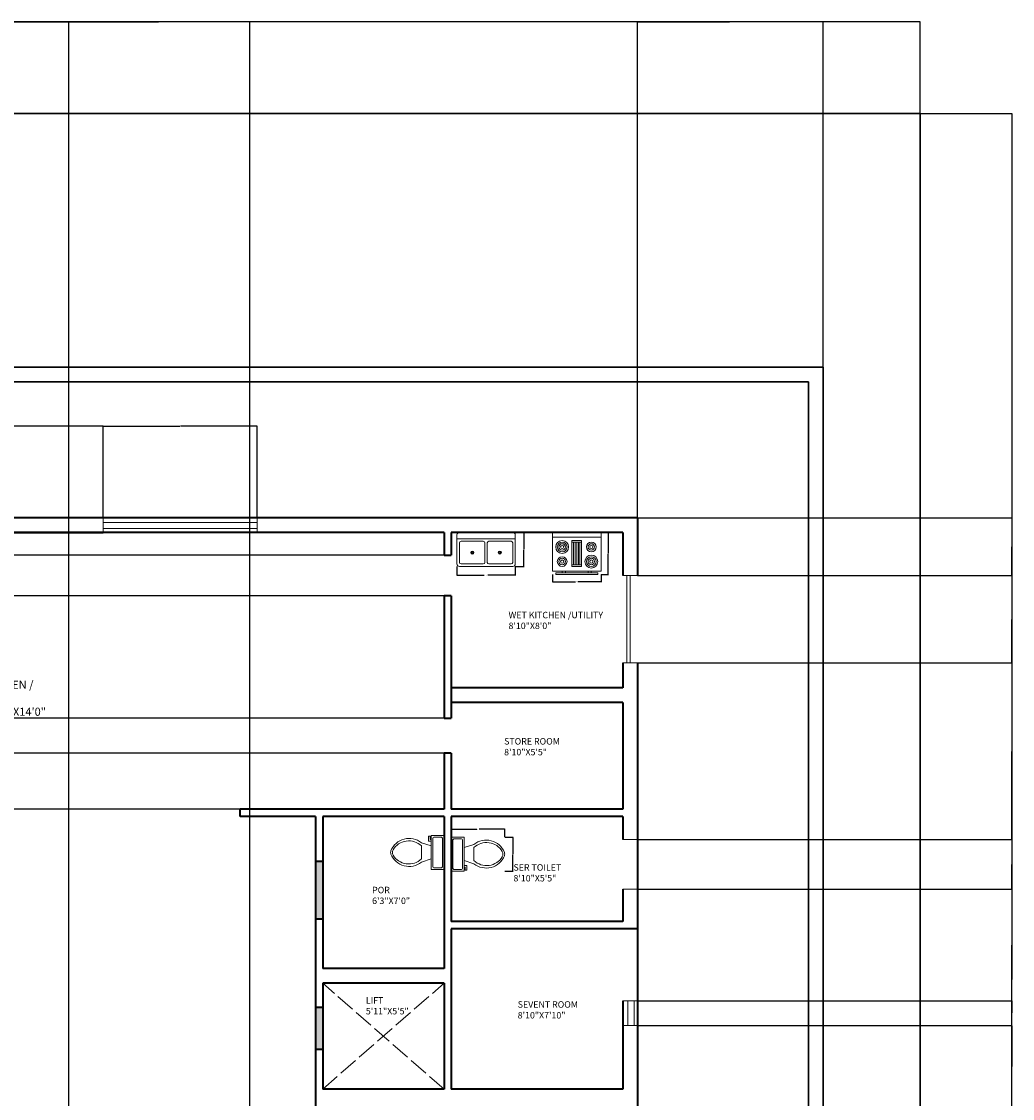
# Model space of a CAD drawing. Units: inches. Extents: x 727 to 1967, y -579 to 606.
# Tile 5 of 5: x 1355 to 1967, y -60 to 606. Entities that reach past the tile are written whole.
import ezdxf

# ---------------------------------------------------------------- set-up
doc = ezdxf.new("R2010")
doc.units = ezdxf.units.IN
doc.header["$MEASUREMENT"] = 0
doc.linetypes.add('ACAD_ISO02W100', pattern=[15, 12, -3])
for name, color, linetype, lineweight in [('A-ANNO-DIMS', 2, 'Continuous', 18), ('A-AREA-IDEN', 7, 'Continuous', 18), ('A-EQPM', 8, 'Continuous', 18), ('A-FLOR-EVTR', 8, 'ACAD_ISO02W100', 18), ('A-FLOR-FIXT', 9, 'Continuous', 18), ('A-GLAZ', 4, 'Continuous', 18), ('A-WALL', 7, 'Continuous', 35), ('A-WALL-PATT', 9, 'Continuous', 13), ('C-PROP', 7, 'Continuous', 30)]:
    doc.layers.add(name, color=color, linetype=linetype, lineweight=lineweight)
doc.styles.get("Standard").update_dxf_attribs({"font": 'arial.ttf'})
doc.dimstyles.get("Standard").update_dxf_attribs({"dimtxt": 0.18, "dimasz": 0.18, "dimexe": 0.18, "dimexo": 0.0625, "dimgap": 0.09, "dimtad": 0, "dimtih": 1, "dimtoh": 1, "dimdec": 4, "dimzin": 0, "dimdsep": 46, "dimtxsty": 'Standard', "dimcen": 0.09, "dimadec": 0, "dimazin": 0, "dimtfac": 1, "dimtdec": 4, "dimtofl": 0, "dimtmove": 0, "dimatfit": 3, "dimfxl": 1, "dimtolj": 1, "dimtzin": 0, "dimarcsym": 0})

# ---------------------------------------------------------------- blocks, each defined once
blk = doc.blocks.new('Range-Oven - 30 in top')
for p, q in [((0, -3), (30, -3)), ((12, -6), (18, -6)), ((13, -20), (13, -6)), ((14, -6), (14, -20)), ((15, -20), (15, -6)), ((16, -6), (16, -20)), ((17, -20), (17, -6)), ((6, -24), (6, -25)), ((8, -25), (8, -24)), ((18, -20), (12, -20)), ((22, -25), (22, -24)), ((24, -24), (24, -25))]:
    blk.add_line(p, q)
for points in [[(0, -24), (0, 0), (30, 0), (30, -24)], [(12, -21), (12, -5), (18, -5), (18, -21)], [(2, -26), (2, -25), (28, -25), (28, -26)]]:
    blk.add_lwpolyline(points, close=True)
for centre, radius in [((6, -9), 4), ((6, -9), 3), ((24, -9), 3), ((6, -9), 2), ((6, -9), 1), ((24, -9), 2), ((24, -9), 1), ((6, -18), 3), ((6, -18), 2), ((6, -18), 1), ((24, -18), 4), ((24, -18), 3), ((24, -18), 2), ((24, -18), 1)]:
    blk.add_circle(centre, radius)
blk = doc.blocks.new('Sink-double - 36 in top')
for p, q in [((-18, -4), (18, -4)), ((-0.75, -18.5), (-0.75, -6.5)), ((0.75, -6.5), (0.75, -18.5))]:
    blk.add_line(p, q)
for points in [[(-16.5, 0), (16.5, 0)], [(-18, -19.5), (-18, -1.5)], [(-16.5, -18.5), (-16.5, -6.5)], [(-15.5, -5.5), (-1.75, -5.5)], [(1.75, -5.5), (15.5, -5.5)], [(16.5, -6.5), (16.5, -18.5)], [(18, -1.5), (18, -19.5)], [(-1.75, -19.5), (-15.5, -19.5)], [(15.5, -19.5), (1.75, -19.5)], [(16.5, -21), (-16.5, -21)]]:
    blk.add_lwpolyline(points)
for centre, radius in [((-8.5, -12.5), 1), ((-8.5, -12.5), 0.5), ((8.5, -12.5), 1), ((8.5, -12.5), 0.5)]:
    blk.add_circle(centre, radius)
for centre, radius, start, end in [((-16.5, -1.5), 1.5, 90, 180), ((16.5, -1.5), 1.5, 0, 90), ((-15.5, -6.5), 1, 90, 180), ((-1.75, -6.5), 1, 0, 90), ((1.75, -6.5), 1, 90, 180), ((15.5, -6.5), 1, 0, 90), ((-16.5, -19.5), 1.5, 180, 270), ((-15.5, -18.5), 1, 180, 270), ((-1.75, -18.5), 1, 270, 0), ((1.75, -18.5), 1, 180, 270), ((15.5, -18.5), 1, 270, 0), ((16.5, -19.5), 1.5, 270, 0)]:
    blk.add_arc(centre, radius, start, end)
blk = doc.blocks.new('Toilet - top')
for p, q in [((9.5, -6), (9.5, -2)), ((-10, -8.5), (-8, -8.5)), ((-10, -9.5), (-10, -8.5)), ((-7, -9.5), (-10, -9.5)), ((-8, -8.5), (-8, -8)), ((-7, -8), (-7, -9.5)), ((-4, -8), (-6, -14)), ((4, -8), (6, -14)), ((4, -14), (-4, -14))]:
    blk.add_line(p, q)
blk.add_lwpolyline([(10.5, -8), (10.5, 0), (-10.5, 0), (-10.5, -8)], close=True)
for points in [[(-9.5, -2), (-9.5, -6)], [(8.5, -1), (-8.5, -1)], [(-8.5, -7), (8.5, -7)]]:
    blk.add_lwpolyline(points)
for centre, radius, start, end in [((-8.62, -1.88), 0.884, 81.8699, 188.1301), ((-8.62, -6.12), 0.884, 171.8699, 278.1301), ((8.62, -1.88), 0.884, 351.8699, 98.1301), ((8.62, -6.12), 0.884, 261.8699, 8.1301), ((3.52, -21.58), 12.17, 141.46911, 247.97143), ((4.2, -21.82), 11.33, 136.36773, 238.94682), ((-3.52, -21.58), 12.17, 292.02843, 38.53071), ((-4.2, -21.82), 11.33, 301.05301, 43.63209), ((0, -27.88), 4, 245.73182, 294.26817), ((0, -29), 4, 254.86053, 285.13947)]:
    blk.add_arc(centre, radius, start, end)
blk = doc.blocks.new('*D20')
at = {"layer": 'A-ANNO-DIMS', "color": 0, "lineweight": -2, "transparency": 16777216}
for p, q in [((1620.35, 101.83), (1620.35, 106.91)), ((1620.53, 106.73), (1636.09, 106.73)), ((1653.21, 106.73), (1637.65, 106.73)), ((1653.39, 101.83), (1653.39, 106.91))]:
    blk.add_line(p, q, dxfattribs=at)
at = {"layer": 'A-ANNO-DIMS', "color": 0, "transparency": 16777216}
for points in [[(1620.53, 106.76), (1620.53, 106.7), (1620.35, 106.73)], [(1653.21, 106.76), (1653.21, 106.7), (1653.39, 106.73)]]:
    blk.add_solid(points, dxfattribs=at)
at = {"layer": 'Defpoints', "color": 0, "transparency": 16777216}
for p in [(1620.35, 106.73), (1620.35, 101.77), (1653.39, 101.77)]:
    blk.add_point(p, dxfattribs=at)
at = {"layer": 'A-ANNO-DIMS', "color": 0, "transparency": 16777216, "insert": (1636.87, 106.73), "char_height": 0.18, "attachment_point": 5}
blk.add_mtext('\\A1;WC 33 TYP.', dxfattribs=at)
blk = doc.blocks.new('*D21')
at = {"layer": 'A-ANNO-DIMS', "color": 0, "lineweight": -2, "transparency": 16777216}
for p, q in [((1653.46, 101.77), (1658.53, 101.77)), ((1658.35, 101.59), (1658.35, 91.45)), ((1658.35, 80.95), (1658.35, 91.09)), ((1653.46, 80.77), (1658.53, 80.77))]:
    blk.add_line(p, q, dxfattribs=at)
at = {"layer": 'A-ANNO-DIMS', "color": 0, "transparency": 16777216}
for points in [[(1658.32, 101.59), (1658.38, 101.59), (1658.35, 101.77)], [(1658.32, 80.95), (1658.38, 80.95), (1658.35, 80.77)]]:
    blk.add_solid(points, dxfattribs=at)
at = {"layer": 'Defpoints', "color": 0, "transparency": 16777216}
for p in [(1653.39, 101.77), (1658.35, 101.77), (1653.39, 80.77)]:
    blk.add_point(p, dxfattribs=at)
at = {"layer": 'A-ANNO-DIMS', "color": 0, "transparency": 16777216, "insert": (1658.35, 91.27), "char_height": 0.18, "attachment_point": 5}
blk.add_mtext('\\A1;21 TYP.', dxfattribs=at)
blk = doc.blocks.new('*D28')
at = {"layer": 'A-ANNO-DIMS', "color": 0, "lineweight": -2, "transparency": 16777216}
for p, q in [((1682.86, 263.95), (1682.86, 259.34)), ((1683.04, 259.52), (1697.17, 259.52)), ((1712.68, 259.52), (1698.56, 259.52)), ((1712.86, 263.95), (1712.86, 259.34))]:
    blk.add_line(p, q, dxfattribs=at)
at = {"layer": 'A-ANNO-DIMS', "color": 0, "transparency": 16777216}
for points in [[(1683.04, 259.55), (1683.04, 259.49), (1682.86, 259.52)], [(1712.68, 259.55), (1712.68, 259.49), (1712.86, 259.52)]]:
    blk.add_solid(points, dxfattribs=at)
at = {"layer": 'Defpoints', "color": 0, "transparency": 16777216}
for p in [(1682.86, 264.02), (1712.86, 264.02), (1712.86, 259.52)]:
    blk.add_point(p, dxfattribs=at)
at = {"layer": 'A-ANNO-DIMS', "color": 0, "transparency": 16777216, "insert": (1697.86, 259.52), "char_height": 0.18, "attachment_point": 5}
blk.add_mtext('\\A1;RANGE 30', dxfattribs=at)
blk = doc.blocks.new('*D29')
at = {"layer": 'A-ANNO-DIMS', "color": 0, "lineweight": -2, "transparency": 16777216}
for p, q in [((1712.93, 290.02), (1717.54, 290.02)), ((1717.36, 289.84), (1717.36, 277.2)), ((1717.36, 264.2), (1717.36, 276.83)), ((1712.93, 264.02), (1717.54, 264.02))]:
    blk.add_line(p, q, dxfattribs=at)
at = {"layer": 'A-ANNO-DIMS', "color": 0, "transparency": 16777216}
for points in [[(1717.33, 289.84), (1717.39, 289.84), (1717.36, 290.02)], [(1717.33, 264.2), (1717.39, 264.2), (1717.36, 264.02)]]:
    blk.add_solid(points, dxfattribs=at)
at = {"layer": 'Defpoints', "color": 0, "transparency": 16777216}
for p in [(1712.86, 290.02), (1717.36, 290.02), (1712.86, 264.02)]:
    blk.add_point(p, dxfattribs=at)
at = {"layer": 'A-ANNO-DIMS', "color": 0, "transparency": 16777216, "insert": (1717.36, 277.02), "char_height": 0.18, "attachment_point": 5}
blk.add_mtext('\\A1;26', dxfattribs=at)
blk = doc.blocks.new('*D30')
at = {"layer": 'A-ANNO-DIMS', "color": 0, "lineweight": -2, "transparency": 16777216}
for p, q in [((1623.85, 268.95), (1623.85, 263.44)), ((1659.85, 268.95), (1659.85, 263.44)), ((1624.03, 263.62), (1640.75, 263.62)), ((1659.67, 263.62), (1642.94, 263.62))]:
    blk.add_line(p, q, dxfattribs=at)
at = {"layer": 'A-ANNO-DIMS', "color": 0, "transparency": 16777216}
for points in [[(1624.03, 263.65), (1624.03, 263.59), (1623.85, 263.62)], [(1659.67, 263.65), (1659.67, 263.59), (1659.85, 263.62)]]:
    blk.add_solid(points, dxfattribs=at)
at = {"layer": 'Defpoints', "color": 0, "transparency": 16777216}
for p in [(1623.85, 269.02), (1659.85, 269.02), (1659.85, 263.62)]:
    blk.add_point(p, dxfattribs=at)
at = {"layer": 'A-ANNO-DIMS', "color": 0, "transparency": 16777216, "insert": (1641.85, 263.62), "char_height": 0.18, "attachment_point": 5}
blk.add_mtext('\\A1;DOUBLE SINK 36', dxfattribs=at)
blk = doc.blocks.new('*D31')
at = {"layer": 'A-ANNO-DIMS', "color": 0, "lineweight": -2, "transparency": 16777216}
for p, q in [((1659.91, 290.02), (1665.43, 290.02)), ((1665.25, 289.84), (1665.25, 279.7)), ((1665.25, 269.2), (1665.25, 279.33)), ((1659.91, 269.02), (1665.43, 269.02))]:
    blk.add_line(p, q, dxfattribs=at)
at = {"layer": 'A-ANNO-DIMS', "color": 0, "transparency": 16777216}
for points in [[(1665.22, 289.84), (1665.28, 289.84), (1665.25, 290.02)], [(1665.22, 269.2), (1665.28, 269.2), (1665.25, 269.02)]]:
    blk.add_solid(points, dxfattribs=at)
at = {"layer": 'Defpoints', "color": 0, "transparency": 16777216}
for p in [(1659.85, 290.02), (1665.25, 290.02), (1659.85, 269.02)]:
    blk.add_point(p, dxfattribs=at)
at = {"layer": 'A-ANNO-DIMS', "color": 0, "transparency": 16777216, "insert": (1665.25, 279.52), "char_height": 0.18, "attachment_point": 5}
blk.add_mtext('\\A1;21', dxfattribs=at)
blk = doc.blocks.new('*D38')
at = {"layer": 'A-ANNO-DIMS', "color": 0, "lineweight": -2, "transparency": 16777216}
for p, q in [((783.58, 548.95), (783.58, 605.67)), ((1910.18, 548.95), (1910.18, 605.67)), ((783.76, 605.49), (1346.42, 605.49)), ((1910, 605.49), (1347.33, 605.49))]:
    blk.add_line(p, q, dxfattribs=at)
at = {"layer": 'A-ANNO-DIMS', "color": 0, "transparency": 16777216}
for points in [[(783.76, 605.52), (783.76, 605.46), (783.58, 605.49)], [(1910, 605.52), (1910, 605.46), (1910.18, 605.49)]]:
    blk.add_solid(points, dxfattribs=at)
at = {"layer": 'Defpoints', "color": 0, "transparency": 16777216}
for p in [(1910.18, 605.49), (783.58, 548.89), (1910.18, 548.89)]:
    blk.add_point(p, dxfattribs=at)
at = {"layer": 'A-ANNO-DIMS', "color": 0, "transparency": 16777216, "insert": (1346.88, 605.49), "char_height": 0.18, "attachment_point": 5}
blk.add_mtext('\\A1;1126.6', dxfattribs=at)
blk = doc.blocks.new('*D39')
at = {"layer": 'A-ANNO-DIMS', "color": 0, "lineweight": -2, "transparency": 16777216}
for p, q in [((1910.24, 548.89), (1966.96, 548.89)), ((1966.78, 548.71), (1966.78, 13.72)), ((1966.78, -521.63), (1966.78, 13.36)), ((1910.24, -521.81), (1966.96, -521.81))]:
    blk.add_line(p, q, dxfattribs=at)
at = {"layer": 'A-ANNO-DIMS', "color": 0, "transparency": 16777216}
for points in [[(1966.75, 548.71), (1966.81, 548.71), (1966.78, 548.89)], [(1966.75, -521.63), (1966.81, -521.63), (1966.78, -521.81)]]:
    blk.add_solid(points, dxfattribs=at)
at = {"layer": 'Defpoints', "color": 0, "transparency": 16777216}
for p in [(1910.18, 548.89), (1966.78, 548.89), (1910.18, -521.81)]:
    blk.add_point(p, dxfattribs=at)
at = {"layer": 'A-ANNO-DIMS', "color": 0, "transparency": 16777216, "insert": (1966.78, 13.54), "char_height": 0.18, "attachment_point": 5}
blk.add_mtext('\\A1;1070.7', dxfattribs=at)
blk = doc.blocks.new('*D42')
at = {"layer": 'A-ANNO-DIMS', "color": 0, "lineweight": -2, "transparency": 16777216}
for p, q in [((1099.85, 299.08), (1099.85, 605.67)), ((1735.35, 299.08), (1735.35, 605.67)), ((1100.03, 605.49), (1417.2, 605.49)), ((1735.17, 605.49), (1417.99, 605.49))]:
    blk.add_line(p, q, dxfattribs=at)
at = {"layer": 'A-ANNO-DIMS', "color": 0, "transparency": 16777216}
for points in [[(1100.03, 605.52), (1100.03, 605.46), (1099.85, 605.49)], [(1735.17, 605.52), (1735.17, 605.46), (1735.35, 605.49)]]:
    blk.add_solid(points, dxfattribs=at)
at = {"layer": 'Defpoints', "color": 0, "transparency": 16777216}
for p in [(1735.35, 605.49), (1099.85, 299.02), (1735.35, 299.02)]:
    blk.add_point(p, dxfattribs=at)
at = {"layer": 'A-ANNO-DIMS', "color": 0, "transparency": 16777216, "insert": (1417.6, 605.49), "char_height": 0.18, "attachment_point": 5}
blk.add_mtext('\\A1;635.5', dxfattribs=at)
blk = doc.blocks.new('*D43')
at = {"layer": 'A-ANNO-DIMS', "color": 0, "lineweight": -2, "transparency": 16777216}
for p, q in [((1735.35, 299.08), (1735.35, 605.67)), ((1850.18, 392.08), (1850.18, 605.67)), ((1735.53, 605.49), (1792.31, 605.49)), ((1850, 605.49), (1793.22, 605.49))]:
    blk.add_line(p, q, dxfattribs=at)
at = {"layer": 'A-ANNO-DIMS', "color": 0, "transparency": 16777216}
for points in [[(1735.53, 605.52), (1735.53, 605.46), (1735.35, 605.49)], [(1850, 605.52), (1850, 605.46), (1850.18, 605.49)]]:
    blk.add_solid(points, dxfattribs=at)
at = {"layer": 'Defpoints', "color": 0, "transparency": 16777216}
for p in [(1850.18, 605.49), (1850.18, 392.02), (1735.35, 299.02)]:
    blk.add_point(p, dxfattribs=at)
at = {"layer": 'A-ANNO-DIMS', "color": 0, "transparency": 16777216, "insert": (1792.76, 605.49), "char_height": 0.18, "attachment_point": 5}
blk.add_mtext('\\A1;114.83', dxfattribs=at)
blk = doc.blocks.new('*D57')
at = {"layer": 'A-ANNO-DIMS', "color": 0, "lineweight": -2, "transparency": 16777216}
for p, q in [((1288.64, 299.08), (1288.64, 355.8)), ((1288.82, 355.62), (1346.51, 355.62)), ((1405.1, 355.62), (1347.42, 355.62)), ((1405.28, 299.08), (1405.28, 355.8))]:
    blk.add_line(p, q, dxfattribs=at)
at = {"layer": 'A-ANNO-DIMS', "color": 0, "transparency": 16777216}
for points in [[(1288.82, 355.65), (1288.82, 355.59), (1288.64, 355.62)], [(1405.1, 355.65), (1405.1, 355.59), (1405.28, 355.62)]]:
    blk.add_solid(points, dxfattribs=at)
at = {"layer": 'Defpoints', "color": 0, "transparency": 16777216}
for p in [(1405.28, 355.62), (1288.64, 299.02), (1405.28, 299.02)]:
    blk.add_point(p, dxfattribs=at)
at = {"layer": 'A-ANNO-DIMS', "color": 0, "transparency": 16777216, "insert": (1346.96, 355.62), "char_height": 0.18, "attachment_point": 5}
blk.add_mtext('\\A1;116.65', dxfattribs=at)
blk = doc.blocks.new('*D58')
at = {"layer": 'A-ANNO-DIMS', "color": 0, "lineweight": -2, "transparency": 16777216}
for p, q in [((1405.28, 299.08), (1405.28, 355.8)), ((1405.46, 355.62), (1452.56, 355.62)), ((1500.1, 355.62), (1453, 355.62)), ((1500.28, 299.08), (1500.28, 355.8))]:
    blk.add_line(p, q, dxfattribs=at)
at = {"layer": 'A-ANNO-DIMS', "color": 0, "transparency": 16777216}
for points in [[(1405.46, 355.65), (1405.46, 355.59), (1405.28, 355.62)], [(1500.1, 355.65), (1500.1, 355.59), (1500.28, 355.62)]]:
    blk.add_solid(points, dxfattribs=at)
at = {"layer": 'Defpoints', "color": 0, "transparency": 16777216}
for p in [(1500.28, 355.62), (1405.28, 299.02), (1500.28, 299.02)]:
    blk.add_point(p, dxfattribs=at)
at = {"layer": 'A-ANNO-DIMS', "color": 0, "transparency": 16777216, "insert": (1452.78, 355.62), "char_height": 0.18, "attachment_point": 5}
blk.add_mtext('\\A1;95', dxfattribs=at)
blk = doc.blocks.new('*D60')
at = {"layer": 'A-ANNO-DIMS', "color": 0, "lineweight": -2, "transparency": 16777216}
for p, q in [((1383.91, -185.42), (1383.91, 605.67)), ((1495.93, -185.42), (1495.93, 605.67)), ((1384.09, 605.49), (1439.47, 605.49)), ((1495.75, 605.49), (1440.38, 605.49))]:
    blk.add_line(p, q, dxfattribs=at)
at = {"layer": 'A-ANNO-DIMS', "color": 0, "transparency": 16777216}
for points in [[(1384.09, 605.52), (1384.09, 605.46), (1383.91, 605.49)], [(1495.75, 605.52), (1495.75, 605.46), (1495.93, 605.49)]]:
    blk.add_solid(points, dxfattribs=at)
at = {"layer": 'Defpoints', "color": 0, "transparency": 16777216}
for p in [(1495.93, 605.49), (1383.91, -185.48), (1495.93, -185.48)]:
    blk.add_point(p, dxfattribs=at)
at = {"layer": 'A-ANNO-DIMS', "color": 0, "transparency": 16777216, "insert": (1439.92, 605.49), "char_height": 0.18, "attachment_point": 5}
blk.add_mtext('\\A1;112.02', dxfattribs=at)
blk = doc.blocks.new('*D61')
at = {"layer": 'A-ANNO-DIMS', "color": 0, "lineweight": -2, "transparency": 16777216}
for p, q in [((1735.41, 299.02), (1966.96, 299.02)), ((1966.78, 298.84), (1966.78, 281.43)), ((1966.78, 263.66), (1966.78, 281.07)), ((1735.41, 263.48), (1966.96, 263.48))]:
    blk.add_line(p, q, dxfattribs=at)
at = {"layer": 'A-ANNO-DIMS', "color": 0, "transparency": 16777216}
for points in [[(1966.75, 298.84), (1966.81, 298.84), (1966.78, 299.02)], [(1966.75, 263.66), (1966.81, 263.66), (1966.78, 263.48)]]:
    blk.add_solid(points, dxfattribs=at)
at = {"layer": 'Defpoints', "color": 0, "transparency": 16777216}
for p in [(1735.35, 299.02), (1735.35, 263.48), (1966.78, 263.48)]:
    blk.add_point(p, dxfattribs=at)
at = {"layer": 'A-ANNO-DIMS', "color": 0, "transparency": 16777216, "insert": (1966.78, 281.25), "char_height": 0.18, "attachment_point": 5}
blk.add_mtext('\\A1;35.534', dxfattribs=at)
blk = doc.blocks.new('*D62')
at = {"layer": 'A-ANNO-DIMS', "color": 0, "lineweight": -2, "transparency": 16777216}
for p, q in [((1735.41, 263.48), (1966.96, 263.48)), ((1966.78, 263.3), (1966.78, 236.6)), ((1966.78, 209.53), (1966.78, 236.24)), ((1735.41, 209.35), (1966.96, 209.35))]:
    blk.add_line(p, q, dxfattribs=at)
at = {"layer": 'A-ANNO-DIMS', "color": 0, "transparency": 16777216}
for points in [[(1966.75, 263.3), (1966.81, 263.3), (1966.78, 263.48)], [(1966.75, 209.53), (1966.81, 209.53), (1966.78, 209.35)]]:
    blk.add_solid(points, dxfattribs=at)
at = {"layer": 'Defpoints', "color": 0, "transparency": 16777216}
for p in [(1735.35, 263.48), (1735.35, 209.35), (1966.78, 209.35)]:
    blk.add_point(p, dxfattribs=at)
at = {"layer": 'A-ANNO-DIMS', "color": 0, "transparency": 16777216, "insert": (1966.78, 236.42), "char_height": 0.18, "attachment_point": 5}
blk.add_mtext('\\A1;54.13', dxfattribs=at)
blk = doc.blocks.new('*D63')
at = {"layer": 'A-ANNO-DIMS', "color": 0, "lineweight": -2, "transparency": 16777216}
for p, q in [((1735.41, 209.35), (1966.96, 209.35)), ((1966.78, 209.17), (1966.78, 155.02)), ((1966.78, 100.51), (1966.78, 154.66)), ((1735.41, 100.33), (1966.96, 100.33))]:
    blk.add_line(p, q, dxfattribs=at)
at = {"layer": 'A-ANNO-DIMS', "color": 0, "transparency": 16777216}
for points in [[(1966.75, 209.17), (1966.81, 209.17), (1966.78, 209.35)], [(1966.75, 100.51), (1966.81, 100.51), (1966.78, 100.33)]]:
    blk.add_solid(points, dxfattribs=at)
at = {"layer": 'Defpoints', "color": 0, "transparency": 16777216}
for p in [(1735.35, 209.35), (1735.35, 100.33), (1966.78, 100.33)]:
    blk.add_point(p, dxfattribs=at)
at = {"layer": 'A-ANNO-DIMS', "color": 0, "transparency": 16777216, "insert": (1966.78, 154.84), "char_height": 0.18, "attachment_point": 5}
blk.add_mtext('\\A1;109.03', dxfattribs=at)
blk = doc.blocks.new('*D64')
at = {"layer": 'A-ANNO-DIMS', "color": 0, "lineweight": -2, "transparency": 16777216}
for p, q in [((1735.41, 100.33), (1966.96, 100.33)), ((1966.78, 100.15), (1966.78, 85.17)), ((1966.78, 69.83), (1966.78, 84.81)), ((1735.41, 69.65), (1966.96, 69.65))]:
    blk.add_line(p, q, dxfattribs=at)
at = {"layer": 'A-ANNO-DIMS', "color": 0, "transparency": 16777216}
for points in [[(1966.75, 100.15), (1966.81, 100.15), (1966.78, 100.33)], [(1966.75, 69.83), (1966.81, 69.83), (1966.78, 69.65)]]:
    blk.add_solid(points, dxfattribs=at)
at = {"layer": 'Defpoints', "color": 0, "transparency": 16777216}
for p in [(1735.35, 100.33), (1735.35, 69.65), (1966.78, 69.65)]:
    blk.add_point(p, dxfattribs=at)
at = {"layer": 'A-ANNO-DIMS', "color": 0, "transparency": 16777216, "insert": (1966.78, 84.99), "char_height": 0.18, "attachment_point": 5}
blk.add_mtext('\\A1;30.67', dxfattribs=at)
blk = doc.blocks.new('*D65')
at = {"layer": 'A-ANNO-DIMS', "color": 0, "lineweight": -2, "transparency": 16777216}
for p, q in [((1735.41, 69.65), (1966.96, 69.65)), ((1966.78, 69.47), (1966.78, 35.35)), ((1966.78, 0.87), (1966.78, 34.99)), ((1735.41, 0.69), (1966.96, 0.69))]:
    blk.add_line(p, q, dxfattribs=at)
at = {"layer": 'A-ANNO-DIMS', "color": 0, "transparency": 16777216}
for points in [[(1966.75, 69.47), (1966.81, 69.47), (1966.78, 69.65)], [(1966.75, 0.87), (1966.81, 0.87), (1966.78, 0.69)]]:
    blk.add_solid(points, dxfattribs=at)
at = {"layer": 'Defpoints', "color": 0, "transparency": 16777216}
for p in [(1735.35, 69.65), (1735.35, 0.69), (1966.78, 0.69)]:
    blk.add_point(p, dxfattribs=at)
at = {"layer": 'A-ANNO-DIMS', "color": 0, "transparency": 16777216, "insert": (1966.78, 35.17), "char_height": 0.18, "attachment_point": 5}
blk.add_mtext('\\A1;68.97', dxfattribs=at)
blk = doc.blocks.new('*D66')
at = {"layer": 'A-ANNO-DIMS', "color": 0, "lineweight": -2, "transparency": 16777216}
for p, q in [((1735.41, 0.69), (1966.96, 0.69)), ((1966.78, 0.51), (1966.78, -6.85)), ((1966.78, -14.57), (1966.78, -7.22)), ((1735.41, -14.75), (1966.96, -14.75))]:
    blk.add_line(p, q, dxfattribs=at)
at = {"layer": 'A-ANNO-DIMS', "color": 0, "transparency": 16777216}
for points in [[(1966.75, 0.51), (1966.81, 0.51), (1966.78, 0.69)], [(1966.75, -14.57), (1966.81, -14.57), (1966.78, -14.75)]]:
    blk.add_solid(points, dxfattribs=at)
at = {"layer": 'Defpoints', "color": 0, "transparency": 16777216}
for p in [(1735.35, 0.69), (1735.35, -14.75), (1966.78, -14.75)]:
    blk.add_point(p, dxfattribs=at)
at = {"layer": 'A-ANNO-DIMS', "color": 0, "transparency": 16777216, "insert": (1966.78, -7.03), "char_height": 0.18, "attachment_point": 5}
blk.add_mtext('\\A1;15.44', dxfattribs=at)
blk = doc.blocks.new('*D67')
at = {"layer": 'A-ANNO-DIMS', "color": 0, "lineweight": -2, "transparency": 16777216}
for p, q in [((1735.41, -14.75), (1966.96, -14.75)), ((1966.78, -14.93), (1966.78, -39.94)), ((1966.78, -65.3), (1966.78, -40.3)), ((1735.41, -65.48), (1966.96, -65.48))]:
    blk.add_line(p, q, dxfattribs=at)
at = {"layer": 'A-ANNO-DIMS', "color": 0, "transparency": 16777216}
for points in [[(1966.75, -14.93), (1966.81, -14.93), (1966.78, -14.75)], [(1966.75, -65.3), (1966.81, -65.3), (1966.78, -65.48)]]:
    blk.add_solid(points, dxfattribs=at)
at = {"layer": 'Defpoints', "color": 0, "transparency": 16777216}
for p in [(1735.35, -14.75), (1735.35, -65.48), (1966.78, -65.48)]:
    blk.add_point(p, dxfattribs=at)
at = {"layer": 'A-ANNO-DIMS', "color": 0, "transparency": 16777216, "insert": (1966.78, -40.12), "char_height": 0.18, "attachment_point": 5}
blk.add_mtext('\\A1;50.73', dxfattribs=at)
blk = doc.blocks.new('*D69')
at = {"layer": 'A-ANNO-DIMS', "color": 0, "lineweight": -2, "transparency": 16777216}
for p, q in [((1615.78, 290.02), (726.8, 290.02)), ((726.98, 289.84), (726.98, 283.18)), ((726.98, 276.17), (726.98, 282.82)), ((1615.78, 275.99), (726.8, 275.99))]:
    blk.add_line(p, q, dxfattribs=at)
at = {"layer": 'A-ANNO-DIMS', "color": 0, "transparency": 16777216}
for points in [[(726.95, 289.84), (727.01, 289.84), (726.98, 290.02)], [(726.95, 276.17), (727.01, 276.17), (726.98, 275.99)]]:
    blk.add_solid(points, dxfattribs=at)
at = {"layer": 'Defpoints', "color": 0, "transparency": 16777216}
for p in [(1615.85, 290.02), (726.98, 275.99), (1615.85, 275.99)]:
    blk.add_point(p, dxfattribs=at)
at = {"layer": 'A-ANNO-DIMS', "color": 0, "transparency": 16777216, "insert": (726.98, 283), "char_height": 0.18, "attachment_point": 5}
blk.add_mtext('\\A1;14.027', dxfattribs=at)
blk = doc.blocks.new('*D70')
at = {"layer": 'A-ANNO-DIMS', "color": 0, "lineweight": -2, "transparency": 16777216}
for p, q in [((1615.78, 275.99), (726.8, 275.99)), ((726.98, 275.81), (726.98, 263.6)), ((726.98, 251.03), (726.98, 263.24)), ((1615.78, 250.85), (726.8, 250.85))]:
    blk.add_line(p, q, dxfattribs=at)
at = {"layer": 'A-ANNO-DIMS', "color": 0, "transparency": 16777216}
for points in [[(726.95, 275.81), (727.01, 275.81), (726.98, 275.99)], [(726.95, 251.03), (727.01, 251.03), (726.98, 250.85)]]:
    blk.add_solid(points, dxfattribs=at)
at = {"layer": 'Defpoints', "color": 0, "transparency": 16777216}
for p in [(1615.85, 275.99), (726.98, 250.85), (1615.85, 250.85)]:
    blk.add_point(p, dxfattribs=at)
at = {"layer": 'A-ANNO-DIMS', "color": 0, "transparency": 16777216, "insert": (726.98, 263.42), "char_height": 0.18, "attachment_point": 5}
blk.add_mtext('\\A1;25.135', dxfattribs=at)
blk = doc.blocks.new('*D71')
at = {"layer": 'A-ANNO-DIMS', "color": 0, "lineweight": -2, "transparency": 16777216}
for p, q in [((1615.78, 250.85), (726.8, 250.85)), ((726.98, 250.67), (726.98, 213.22)), ((726.98, 175.39), (726.98, 212.85)), ((1615.78, 175.21), (726.8, 175.21))]:
    blk.add_line(p, q, dxfattribs=at)
at = {"layer": 'A-ANNO-DIMS', "color": 0, "transparency": 16777216}
for points in [[(726.95, 250.67), (727.01, 250.67), (726.98, 250.85)], [(726.95, 175.39), (727.01, 175.39), (726.98, 175.21)]]:
    blk.add_solid(points, dxfattribs=at)
at = {"layer": 'Defpoints', "color": 0, "transparency": 16777216}
for p in [(1615.85, 250.85), (726.98, 175.21), (1615.85, 175.21)]:
    blk.add_point(p, dxfattribs=at)
at = {"layer": 'A-ANNO-DIMS', "color": 0, "transparency": 16777216, "insert": (726.98, 213.03), "char_height": 0.18, "attachment_point": 5}
blk.add_mtext('\\A1;75.64', dxfattribs=at)
blk = doc.blocks.new('*D72')
at = {"layer": 'A-ANNO-DIMS', "color": 0, "lineweight": -2, "transparency": 16777216}
for p, q in [((1615.78, 175.21), (726.8, 175.21)), ((726.98, 175.03), (726.98, 164.56)), ((726.98, 153.73), (726.98, 164.2)), ((1615.78, 153.55), (726.8, 153.55))]:
    blk.add_line(p, q, dxfattribs=at)
at = {"layer": 'A-ANNO-DIMS', "color": 0, "transparency": 16777216}
for points in [[(726.95, 175.03), (727.01, 175.03), (726.98, 175.21)], [(726.95, 153.73), (727.01, 153.73), (726.98, 153.55)]]:
    blk.add_solid(points, dxfattribs=at)
at = {"layer": 'Defpoints', "color": 0, "transparency": 16777216}
for p in [(1615.85, 175.21), (726.98, 153.55), (1615.85, 153.55)]:
    blk.add_point(p, dxfattribs=at)
at = {"layer": 'A-ANNO-DIMS', "color": 0, "transparency": 16777216, "insert": (726.98, 164.38), "char_height": 0.18, "attachment_point": 5}
blk.add_mtext('\\A1;21.67', dxfattribs=at)
blk = doc.blocks.new('*D73')
at = {"layer": 'A-ANNO-DIMS', "color": 0, "lineweight": -2, "transparency": 16777216}
for p, q in [((1615.78, 153.55), (726.8, 153.55)), ((726.98, 153.37), (726.98, 136.46)), ((726.98, 119.2), (726.98, 136.1)), ((1615.78, 119.02), (726.8, 119.02))]:
    blk.add_line(p, q, dxfattribs=at)
at = {"layer": 'A-ANNO-DIMS', "color": 0, "transparency": 16777216}
for points in [[(726.95, 153.37), (727.01, 153.37), (726.98, 153.55)], [(726.95, 119.2), (727.01, 119.2), (726.98, 119.02)]]:
    blk.add_solid(points, dxfattribs=at)
at = {"layer": 'Defpoints', "color": 0, "transparency": 16777216}
for p in [(1615.85, 153.55), (726.98, 119.02), (1615.85, 119.02)]:
    blk.add_point(p, dxfattribs=at)
at = {"layer": 'A-ANNO-DIMS', "color": 0, "transparency": 16777216, "insert": (726.98, 136.28), "char_height": 0.18, "attachment_point": 5}
blk.add_mtext('\\A1;34.53', dxfattribs=at)

msp = doc.modelspace()

# ---------------------------------------------------------------- hatches: boundary and pattern name
at = {"layer": 'A-WALL-PATT'}
h = msp.add_hatch(color=256, dxfattribs=at)
h.dxf.hatch_style = 1
h.paths.add_polyline_path([(1536.3463, 51.1439), (1540.8463, 51.1439), (1540.8463, 86.7969), (1536.3463, 86.7969)])
h.paths.add_polyline_path([(1536.3463, -29.217), (1540.8463, -29.217), (1540.8463, -3.5401), (1536.3463, -3.5401)])

# ---------------------------------------------------------------- linework, layer by layer
at = {"layer": 'A-FLOR-EVTR'}
for p, q in [((1540.8463, -53.9849), (1615.8463, 11.5151)), ((1615.8463, -53.9849), (1540.8463, 11.5151))]:
    msp.add_line(p, q, dxfattribs=at)
at = {"layer": 'A-GLAZ'}
for p, q in [((1405.2835, 290.0151), (1405.2835, 299.0151)), ((1405.2835, 299.0151), (1500.2781, 299.0151)), ((1405.2835, 292.5171), (1405.2835, 296.1248)), ((1405.2835, 296.1248), (1500.2781, 296.1248)), ((1500.2781, 299.0151), (1500.2781, 290.0151)), ((1500.2781, 292.5171), (1405.2835, 292.5171)), ((1500.2781, 290.0151), (1500.2781, 292.5171)), ((1735.3463, 263.4809), (1726.3463, 263.4809)), ((1728.876, 263.4809), (1728.876, 209.3543)), ((1730.8463, 209.3543), (1730.8463, 263.4809)), ((1726.3463, 209.3543), (1735.3463, 209.3543)), ((1728.876, 209.3543), (1730.8463, 209.3543)), ((1726.3463, 100.3256), (1735.3463, 100.3256)), ((1735.3463, 100.3256), (1735.3463, 69.6534)), ((1735.3463, 69.6534), (1726.3463, 69.6534)), ((1735.3463, 0.6867), (1726.3463, 0.6867)), ((1726.3463, 0.6867), (1729.3906, 0.6867)), ((1729.3906, 0.6867), (1729.3906, -14.7535)), ((1733.3452, -14.7535), (1733.3452, 0.6867)), ((1733.3452, 0.6867), (1735.3463, 0.6867)), ((1726.3463, -14.7535), (1733.3452, -14.7535)), ((1733.3452, -14.7535), (1735.3463, -14.7535)), ((1735.3463, -14.7535), (1733.3452, -14.7535))]:
    msp.add_line(p, q, dxfattribs=at)
at = {"layer": 'A-WALL'}
for p, q in [((1735.3463, 299.0151), (1288.6382, 299.0151)), ((1735.3463, 299.0151), (1735.3463, 263.4809)), ((1615.8463, 290.0151), (1283.8463, 290.0151)), ((1345.2945, 290.0151), (1405.2835, 290.0151)), ((1615.8463, 290.0151), (1615.8463, 275.988)), ((1620.3463, 290.0151), (1620.3463, 275.988)), ((1726.3463, 290.0151), (1620.3463, 290.0151)), ((1726.3463, 290.0151), (1726.3463, 263.4809)), ((1615.8463, 275.988), (1620.3463, 275.988)), ((1620.3463, 250.8534), (1615.8463, 250.8534)), ((1615.8463, 250.8534), (1615.8463, 175.2149)), ((1620.3463, 250.8534), (1620.3463, 175.2149)), ((1726.3463, 209.3543), (1726.3463, 194.0151)), ((1735.3463, 209.3543), (1735.3463, -146.0061)), ((1726.3463, 194.0151), (1620.3463, 194.0151)), ((1726.3463, 185.0151), (1620.3463, 185.0151)), ((1726.3463, 185.0151), (1726.3463, 119.0151)), ((1615.8463, 175.2149), (1620.3463, 175.2149)), ((1620.3463, 153.5464), (1615.8463, 153.5464)), ((1615.8463, 153.5464), (1615.8463, 119.0151)), ((1620.3463, 153.5464), (1620.3463, 119.0151)), ((1489.8185, 114.5151), (1489.8185, 119.0151)), ((1615.8463, 119.0151), (1489.8185, 119.0151)), ((1536.3463, 114.5151), (1489.8185, 114.5151)), ((1536.3463, 114.5151), (1536.3463, -65.4849)), ((1615.8463, 114.5151), (1540.8463, 114.5151)), ((1540.8463, 114.5151), (1540.8463, 20.5151)), ((1615.8463, 114.5151), (1615.8463, 20.5151)), ((1726.3463, 119.0151), (1620.3463, 119.0151)), ((1726.3463, 114.5151), (1620.3463, 114.5151)), ((1620.3463, 114.5151), (1620.3463, 49.5151)), ((1726.3463, 114.5151), (1726.3463, 100.3256)), ((1536.3463, 86.7969), (1540.8463, 86.7969)), ((1540.8463, 86.7969), (1540.8463, 51.1439)), ((1726.3463, 69.6534), (1726.3463, 49.5151)), ((1540.8463, 51.1439), (1536.3463, 51.1439)), ((1726.3463, 49.5151), (1620.3463, 49.5151)), ((1735.3463, 45.0151), (1620.3463, 45.0151)), ((1620.3463, 45.0151), (1620.3463, -53.9849)), ((1615.8463, 20.5151), (1540.8463, 20.5151)), ((1615.8463, 11.5151), (1540.8463, 11.5151)), ((1540.8463, 11.5151), (1540.8463, -53.9849)), ((1615.8463, 11.5151), (1615.8463, -53.9849)), ((1726.3463, 0.6867), (1726.3463, -53.9849)), ((1540.8463, -3.5401), (1536.3463, -3.5401)), ((1536.3463, -3.5401), (1536.3463, -29.217)), ((1536.3463, -29.217), (1540.8463, -29.217)), ((1615.8463, -53.9849), (1540.8463, -53.9849)), ((1726.3463, -53.9849), (1620.3463, -53.9849))]:
    msp.add_line(p, q, dxfattribs=at)
at = {"layer": 'C-PROP'}
for p, q in [((783.5815, 548.8891), (1910.1781, 548.8891)), ((1910.1781, 548.8891), (1910.1781, -521.8103)), ((843.5815, 392.0151), (1850.1781, 392.0151)), ((1850.1781, 392.0151), (1850.1781, -521.8103)), ((852.5815, 383.0151), (1841.1781, 383.0151)), ((1841.1781, 383.0151), (1841.1781, -512.8103))]:
    msp.add_line(p, q, dxfattribs=at)

# ---------------------------------------------------------------- block references
at = {"layer": 'A-EQPM'}
msp.add_blockref('Range-Oven - 30 in top', (1682.8639, 290.0151), dxfattribs=at)
at = {"layer": 'A-FLOR-FIXT'}
msp.add_blockref('Sink-double - 36 in top', (1641.8465, 290.0151), dxfattribs=at)
for p, rotation in [((1615.8463, 92.2768), 270.0000413122306), ((1620.3463, 91.2684), 90.00004131223059)]:
    msp.add_blockref('Toilet - top', p, dxfattribs=dict(at, rotation=rotation))

# ---------------------------------------------------------------- texts
at = {"layer": 'A-AREA-IDEN', "attachment_point": 1}
for s, insert, char_height in [('WET KITCHEN /UTILITY\\P8\'10"X8\'0"', (1655.7221, 240.9587), 4), ('KITCHEN /\\PLIVING\\P26\'11"X14\'0"', (1329.1678, 198.3978), 5), ('STORE ROOM\\P8\'10"X5\'5"', (1652.9917, 162.9303), 4), ('SER TOILET\\P8\'10"X5\'5"', (1658.7648, 85.0227), 4), ('POR\\P6\'3"X7\'0"', (1571.4067, 71.0562), 4), ('LIFT\\P5\'11"X5\'5"', (1567.5356, 2.862), 4), ('SEVENT ROOM\\P8\'10"X7\'10"', (1661.3856, 0.351), 4)]:
    msp.add_mtext_dynamic_manual_height_columns(s, width=588.620786, gutter_width=1, heights=[0], dxfattribs=dict(at, insert=insert, char_height=char_height))

# ---------------------------------------------------------------- dimensions: what is measured, and where the dimension line sits
at = {"layer": 'A-ANNO-DIMS'}
for base, p1, p2, override, picture, middle in [((1910.1781, 605.4891), (783.5815, 548.8891), (1910.1781, 548.8891), {"dimdec": 1, "dimlfac": 1, "dimrnd": 0, "dimzin": 0, "dimdsep": 46, "dimlunit": 2}, '*D38', (1346.8798, 605.4891)), ((1735.3463, 605.4891), (1099.8463, 299.0151), (1735.3463, 299.0151), {"dimdec": 1, "dimlfac": 1, "dimrnd": 0, "dimzin": 0, "dimdsep": 46, "dimlunit": 2}, '*D42', (1417.5963, 605.4891)), ((1495.9329, 605.4891), (1383.9141, -185.4849), (1495.9329, -185.4849), {"dimdec": 2, "dimlfac": 1, "dimrnd": 0, "dimzin": 0, "dimdsep": 46, "dimlunit": 2}, '*D60', (1439.9235, 605.4891)), ((1850.1781, 605.4891), (1735.3463, 299.0151), (1850.1781, 392.0151), {"dimdec": 2, "dimlfac": 1, "dimrnd": 0, "dimzin": 0, "dimdsep": 46, "dimlunit": 2}, '*D43', (1792.7622, 605.4891)), ((1405.2835, 355.6151), (1288.6382, 299.0151), (1405.2835, 299.0151), {"dimdec": 2, "dimlfac": 1, "dimrnd": 0, "dimzin": 0, "dimdsep": 46, "dimlunit": 2}, '*D57', (1346.9609, 355.6151)), ((1500.2781, 355.6151), (1405.2835, 299.0151), (1500.2781, 299.0151), {"dimdec": 0, "dimlfac": 1, "dimrnd": 0, "dimzin": 0, "dimdsep": 46, "dimlunit": 2}, '*D58', (1452.7808, 355.6151))]:
    dim = msp.add_linear_dim(base=base, p1=p1, p2=p2, dimstyle='Standard', override=override, dxfattribs=at)
    dim.commit()
    dim.dimension.update_dxf_attribs({"geometry": picture, "text_midpoint": middle})
for base, p1, p2, override, picture, middle in [((1966.7781, 548.8891), (1910.1781, -521.8103), (1910.1781, 548.8891), {"dimdec": 1, "dimlfac": 1, "dimrnd": 0, "dimzin": 0, "dimdsep": 46, "dimlunit": 2}, '*D39', (1966.7781, 13.5394)), ((1966.7781, 263.4809), (1735.3463, 299.0151), (1735.3463, 263.4809), {"dimdec": 3, "dimlfac": 1, "dimrnd": 0, "dimzin": 0, "dimdsep": 46, "dimlunit": 2}, '*D61', (1966.7781, 281.248)), ((726.9815, 275.988), (1615.8463, 290.0151), (1615.8463, 275.988), {"dimdec": 3, "dimlfac": 1, "dimrnd": 0, "dimzin": 0, "dimdsep": 46, "dimlunit": 2}, '*D69', (726.9815, 283.0015)), ((1665.2465, 290.0151), (1659.8465, 269.0151), (1659.8465, 290.0151), {"dimdec": 0, "dimlfac": 1, "dimrnd": 0, "dimzin": 0, "dimdsep": 46, "dimlunit": 2}, '*D31', (1665.2465, 279.5151)), ((1717.3639, 290.0151), (1712.8639, 264.0151), (1712.8639, 290.0151), {"dimdec": 0, "dimlfac": 1, "dimrnd": 0, "dimzin": 0, "dimdsep": 46, "dimlunit": 2}, '*D29', (1717.3639, 277.0151)), ((726.9815, 250.8534), (1615.8463, 275.988), (1615.8463, 250.8534), {"dimdec": 3, "dimlfac": 1, "dimrnd": 0, "dimzin": 0, "dimdsep": 46, "dimlunit": 2}, '*D70', (726.9815, 263.4207)), ((1966.7781, 209.3543), (1735.3463, 263.4809), (1735.3463, 209.3543), {"dimdec": 2, "dimlfac": 1, "dimrnd": 0, "dimzin": 0, "dimdsep": 46, "dimlunit": 2}, '*D62', (1966.7781, 236.4176)), ((726.9815, 175.2149), (1615.8463, 250.8534), (1615.8463, 175.2149), {"dimdec": 2, "dimlfac": 1, "dimrnd": 0, "dimzin": 0, "dimdsep": 46, "dimlunit": 2}, '*D71', (726.9815, 213.0341)), ((1966.7781, 100.3256), (1735.3463, 209.3543), (1735.3463, 100.3256), {"dimdec": 2, "dimlfac": 1, "dimrnd": 0, "dimzin": 0, "dimdsep": 46, "dimlunit": 2}, '*D63', (1966.7781, 154.8399)), ((726.9815, 153.5464), (1615.8463, 175.2149), (1615.8463, 153.5464), {"dimdec": 2, "dimlfac": 1, "dimrnd": 0, "dimzin": 0, "dimdsep": 46, "dimlunit": 2}, '*D72', (726.9815, 164.3806)), ((726.9815, 119.0151), (1615.8463, 153.5464), (1615.8463, 119.0151), {"dimdec": 2, "dimlfac": 1, "dimrnd": 0, "dimzin": 0, "dimdsep": 46, "dimlunit": 2}, '*D73', (726.9815, 136.2808)), ((1966.7781, 69.6534), (1735.3463, 100.3256), (1735.3463, 69.6534), {"dimdec": 2, "dimlfac": 1, "dimrnd": 0, "dimzin": 0, "dimdsep": 46, "dimlunit": 2}, '*D64', (1966.7781, 84.9895)), ((1966.7781, 0.6867), (1735.3463, 69.6534), (1735.3463, 0.6867), {"dimdec": 2, "dimlfac": 1, "dimrnd": 0, "dimzin": 0, "dimdsep": 46, "dimlunit": 2}, '*D65', (1966.7781, 35.1701)), ((1966.7781, -14.7535), (1735.3463, 0.6867), (1735.3463, -14.7535), {"dimdec": 2, "dimlfac": 1, "dimrnd": 0, "dimzin": 0, "dimdsep": 46, "dimlunit": 2}, '*D66', (1966.7781, -7.0334)), ((1966.7781, -65.4849), (1735.3463, -14.7535), (1735.3463, -65.4849), {"dimdec": 2, "dimlfac": 1, "dimrnd": 0, "dimzin": 0, "dimdsep": 46, "dimlunit": 2}, '*D67', (1966.7781, -40.1192))]:
    dim = msp.add_linear_dim(base=base, p1=p1, p2=p2, angle=90, dimstyle='Standard', override=override, dxfattribs=at)
    dim.commit()
    dim.dimension.update_dxf_attribs({"geometry": picture, "text_midpoint": middle})
for base, p1, p2, text, picture, middle in [((1659.8465, 263.6151), (1623.8465, 269.0151), (1659.8465, 269.0151), 'DOUBLE SINK <>', '*D30', (1641.8465, 263.6151)), ((1712.8639, 259.5151), (1682.8639, 264.0151), (1712.8639, 264.0151), 'RANGE <>', '*D28', (1697.8639, 259.5151))]:
    dim = msp.add_linear_dim(base=base, p1=p1, p2=p2, text=text, dimstyle='Standard', override={"dimdec": 0, "dimlfac": 1, "dimrnd": 0, "dimzin": 0, "dimdsep": 46, "dimlunit": 2}, dxfattribs=at)
    dim.commit()
    dim.dimension.update_dxf_attribs({"geometry": picture, "text_midpoint": middle})
for base, p1, p2, angle, text, picture, middle in [((1620.3463, 106.7253), (1653.3925, 101.7684), (1620.3463, 101.7684), 180.0000413, 'WC <> TYP.', '*D20', (1636.8694, 106.7253)), ((1658.3495, 101.7684), (1653.3925, 80.7684), (1653.3925, 101.7684), 90.0000413, '<> TYP.', '*D21', (1658.3495, 91.2684))]:
    dim = msp.add_linear_dim(base=base, p1=p1, p2=p2, angle=angle, text=text, dimstyle='Standard', override={"dimdec": 0, "dimlfac": 1, "dimrnd": 0, "dimzin": 0, "dimdsep": 46, "dimlunit": 2}, dxfattribs=at)
    dim.commit()
    dim.dimension.update_dxf_attribs({"geometry": picture, "text_midpoint": middle})

doc.saveas('drawing.dxf')
